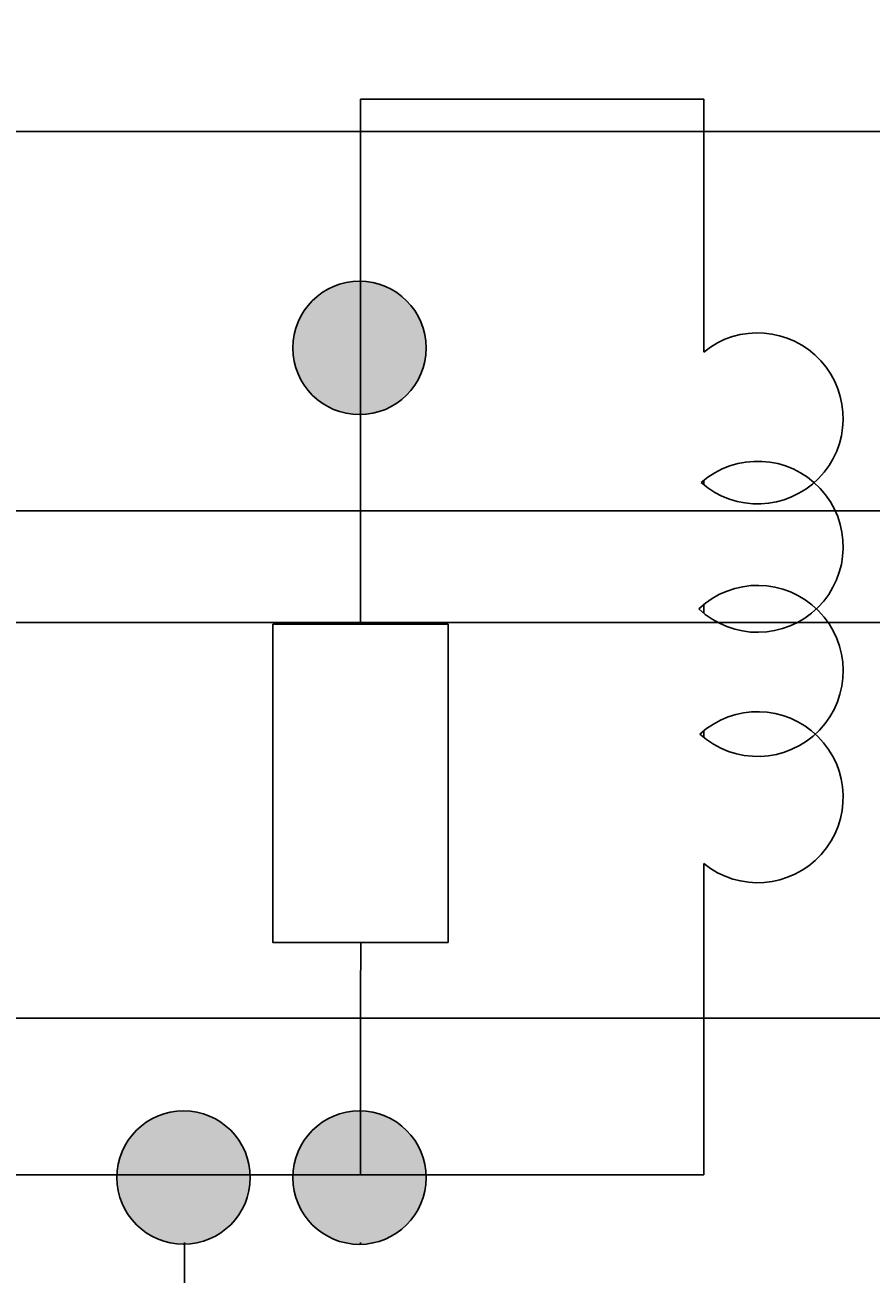
# Model space of a CAD drawing. Units: inches. Extents: x 35362 to 73946, y 43607 to 67532.
# Tile 134 of 134: x 69338 to 71350, y 58575 to 61547. Entities that reach past the tile are written whole.
import ezdxf

# ---------------------------------------------------------------- set-up
doc = ezdxf.new("R2010")
doc.units = ezdxf.units.IN
doc.header["$MEASUREMENT"] = 0
for name, color, linetype, lineweight in [('A-ANNO-DIMS', 2, 'Continuous', 18), ('E-SYMB', 1, 'Continuous', 25), ('E-SYMB-PATT', 1, 'Continuous', 13), ('E-WIRE', 3, 'Continuous', 25)]:
    doc.layers.add(name, color=color, linetype=linetype, lineweight=lineweight)
doc.styles.get("Standard").update_dxf_attribs({"font": 'arial.ttf'})
doc.dimstyles.get("Standard").update_dxf_attribs({"dimtxt": 0.18, "dimasz": 0.18, "dimexe": 0.18, "dimexo": 0.0625, "dimgap": 0.09, "dimtad": 0, "dimtih": 1, "dimtoh": 1, "dimdec": 4, "dimzin": 0, "dimdsep": 46, "dimtxsty": 'Standard', "dimcen": 0.09, "dimadec": 0, "dimazin": 0, "dimtfac": 1, "dimtdec": 4, "dimtofl": 0, "dimtmove": 0, "dimatfit": 3, "dimfxl": 1, "dimtolj": 1, "dimtzin": 0, "dimarcsym": 0})

# ---------------------------------------------------------------- blocks, each defined once
blk = doc.blocks.new('*D8')
at = {"layer": 'A-ANNO-DIMS', "color": 0, "lineweight": -2, "transparency": 16777216}
for p, q in [((66271.28651900003, 65771.51172800003), (73945.82566600003, 65771.51172800003)), ((73945.64566600005, 65771.33172800003), (73945.64566600005, 59737.03093663782)), ((73945.64566600005, 53702.36633900002), (73945.64566600005, 59736.66713036224)), ((72185.70816600003, 53702.18633900003), (73945.82566600003, 53702.18633900003))]:
    blk.add_line(p, q, dxfattribs=at)
at = {"layer": 'A-ANNO-DIMS', "color": 0, "transparency": 16777216}
for points in [[(73945.61566600006, 65771.33172800003), (73945.67566600005, 65771.33172800003), (73945.64566600005, 65771.51172800003)], [(73945.61566600006, 53702.36633900002), (73945.67566600005, 53702.36633900002), (73945.64566600005, 53702.18633900003)]]:
    blk.add_solid(points, dxfattribs=at)
at = {"layer": 'Defpoints', "color": 0, "transparency": 16777216}
for p in [(66271.22401900003, 65771.51172800003), (73945.64566600005, 65771.51172800003), (72185.64566600003, 53702.18633900003)]:
    blk.add_point(p, dxfattribs=at)
at = {"layer": 'A-ANNO-DIMS', "color": 0, "transparency": 16777216, "insert": (73945.64566600005, 59736.84903349999), "char_height": 0.18, "attachment_point": 5}
blk.add_mtext('\\A1;12069', dxfattribs=at)
blk = doc.blocks.new('*D10')
at = {"layer": 'A-ANNO-DIMS', "color": 0, "lineweight": -2, "transparency": 16777216}
for p, q in [((61240.96983600002, 59185.14395700003), (73945.82566600003, 59185.14395700003)), ((73945.64566600005, 59184.96395700003), (73945.64566600005, 56268.51827402935)), ((73945.64566600005, 53351.70866200003), (73945.64566600005, 56268.1543449707)), ((61240.96983600002, 53351.52866200003), (73945.82566600003, 53351.52866200003))]:
    blk.add_line(p, q, dxfattribs=at)
at = {"layer": 'A-ANNO-DIMS', "color": 0, "transparency": 16777216}
for points in [[(73945.61566600006, 59184.96395700003), (73945.67566600005, 59184.96395700003), (73945.64566600005, 59185.14395700003)], [(73945.61566600006, 53351.70866200003), (73945.67566600005, 53351.70866200003), (73945.64566600005, 53351.52866200003)]]:
    blk.add_solid(points, dxfattribs=at)
at = {"layer": 'Defpoints', "color": 0, "transparency": 16777216}
for p in [(61240.90733600002, 59185.14395700003), (61240.90733600002, 53351.52866200003), (73945.64566600005, 53351.52866200003)]:
    blk.add_point(p, dxfattribs=at)
at = {"layer": 'A-ANNO-DIMS', "color": 0, "transparency": 16777216, "insert": (73945.64566600005, 56268.33630949999), "char_height": 0.18, "attachment_point": 5}
blk.add_mtext('\\A1;5834', dxfattribs=at)
blk = doc.blocks.new('*D66')
at = {"layer": 'A-ANNO-DIMS', "color": 0, "lineweight": -2, "transparency": 16777216}
for p, q in [((67326.70224100004, 64127.44160800003), (73945.82566600003, 64127.44160800003)), ((73945.64566600005, 64127.26160800003), (73945.64566600005, 62710.54579452936)), ((73945.64566600005, 61293.46605200003), (73945.64566600005, 62710.1818654707)), ((67326.70224100004, 61293.28605200003), (73945.82566600003, 61293.28605200003))]:
    blk.add_line(p, q, dxfattribs=at)
at = {"layer": 'A-ANNO-DIMS', "color": 0, "transparency": 16777216}
for points in [[(73945.61566600006, 64127.26160800003), (73945.67566600005, 64127.26160800003), (73945.64566600005, 64127.44160800003)], [(73945.61566600006, 61293.46605200003), (73945.67566600005, 61293.46605200003), (73945.64566600005, 61293.28605200003)]]:
    blk.add_solid(points, dxfattribs=at)
at = {"layer": 'Defpoints', "color": 0, "transparency": 16777216}
for p in [(67326.63974100004, 64127.44160800003), (73945.64566600005, 64127.44160800003), (67326.63974100004, 61293.28605200003)]:
    blk.add_point(p, dxfattribs=at)
at = {"layer": 'A-ANNO-DIMS', "color": 0, "transparency": 16777216, "insert": (73945.64566600005, 62710.36383), "char_height": 0.18, "attachment_point": 5}
blk.add_mtext('\\A1;2834.2', dxfattribs=at)
blk = doc.blocks.new('*D69')
at = {"layer": 'A-ANNO-DIMS', "color": 0, "lineweight": -2, "transparency": 16777216}
for p, q in [((68320.870762, 60122.408832), (68320.870762, 67531.691728)), ((68321.050762, 67531.51172799998), (69913.30289879469, 67531.51172799998)), ((71506.482539, 67531.51172799998), (69914.23040220531, 67531.51172799998)), ((71506.662539, 59451.647447), (71506.662539, 67531.691728))]:
    blk.add_line(p, q, dxfattribs=at)
at = {"layer": 'A-ANNO-DIMS', "color": 0, "transparency": 16777216}
for points in [[(68321.050762, 67531.541728), (68321.050762, 67531.481728), (68320.870762, 67531.51172799998)], [(71506.482539, 67531.541728), (71506.482539, 67531.481728), (71506.662539, 67531.51172799998)]]:
    blk.add_solid(points, dxfattribs=at)
at = {"layer": 'Defpoints', "color": 0, "transparency": 16777216}
for p in [(71506.662539, 67531.51172799998), (68320.870762, 60122.346332), (71506.662539, 59451.584947)]:
    blk.add_point(p, dxfattribs=at)
at = {"layer": 'A-ANNO-DIMS', "color": 0, "transparency": 16777216, "insert": (69913.76665050001, 67531.51172799998), "char_height": 0.18, "attachment_point": 5}
blk.add_mtext('\\A1;3185.8', dxfattribs=at)
blk = doc.blocks.new('*D70')
at = {"layer": 'A-ANNO-DIMS', "color": 0, "lineweight": -2, "transparency": 16777216}
for p, q in [((60785.27513900002, 64923.75242000003), (73945.82566600003, 64923.75242000003)), ((73945.64566600005, 64923.57242000003), (73945.64566600005, 62054.63015302935)), ((73945.64566600005, 59185.32395700003), (73945.64566600005, 62054.26622397069)), ((61240.96983600002, 59185.14395700003), (73945.82566600003, 59185.14395700003))]:
    blk.add_line(p, q, dxfattribs=at)
at = {"layer": 'A-ANNO-DIMS', "color": 0, "transparency": 16777216}
for points in [[(73945.61566600006, 64923.57242000003), (73945.67566600005, 64923.57242000003), (73945.64566600005, 64923.75242000003)], [(73945.61566600006, 59185.32395700003), (73945.67566600005, 59185.32395700003), (73945.64566600005, 59185.14395700003)]]:
    blk.add_solid(points, dxfattribs=at)
at = {"layer": 'Defpoints', "color": 0, "transparency": 16777216}
for p in [(60785.21263900002, 64923.75242000003), (73945.64566600005, 64923.75242000003), (61240.90733600002, 59185.14395700003)]:
    blk.add_point(p, dxfattribs=at)
at = {"layer": 'A-ANNO-DIMS', "color": 0, "transparency": 16777216, "insert": (73945.64566600005, 62054.44818849999), "char_height": 0.18, "attachment_point": 5}
blk.add_mtext('\\A1;5738.6', dxfattribs=at)
blk = doc.blocks.new('*D71')
at = {"layer": 'A-ANNO-DIMS', "color": 0, "lineweight": -2, "transparency": 16777216}
for p, q in [((63159.24181700003, 64828.55626700002), (73945.82566600003, 64828.55626700002)), ((73945.64566600005, 64828.37626700002), (73945.64566600005, 62007.03207652936)), ((73945.64566600005, 59185.32395700003), (73945.64566600005, 62006.6681474707)), ((61240.96983600002, 59185.14395700003), (73945.82566600003, 59185.14395700003))]:
    blk.add_line(p, q, dxfattribs=at)
at = {"layer": 'A-ANNO-DIMS', "color": 0, "transparency": 16777216}
for points in [[(73945.61566600006, 64828.37626700002), (73945.67566600005, 64828.37626700002), (73945.64566600005, 64828.55626700002)], [(73945.61566600006, 59185.32395700003), (73945.67566600005, 59185.32395700003), (73945.64566600005, 59185.14395700003)]]:
    blk.add_solid(points, dxfattribs=at)
at = {"layer": 'Defpoints', "color": 0, "transparency": 16777216}
for p in [(63159.17931700003, 64828.55626700002), (73945.64566600005, 64828.55626700002), (61240.90733600002, 59185.14395700003)]:
    blk.add_point(p, dxfattribs=at)
at = {"layer": 'A-ANNO-DIMS', "color": 0, "transparency": 16777216, "insert": (73945.64566600005, 62006.85011199999), "char_height": 0.18, "attachment_point": 5}
blk.add_mtext('\\A1;5643.4', dxfattribs=at)
blk = doc.blocks.new('*D113')
at = {"layer": 'A-ANNO-DIMS', "color": 0, "lineweight": -2, "transparency": 16777216}
for p, q in [((53526.13474100003, 60391.71935800003), (73945.82566600003, 60391.71935800003)), ((73945.64566600005, 60391.53935800003), (73945.64566600005, 60259.19182863781)), ((73945.64566600005, 60126.48049300003), (73945.64566600005, 60258.82802236224)), ((53705.42262200003, 60126.30049300003), (73945.82566600003, 60126.30049300003))]:
    blk.add_line(p, q, dxfattribs=at)
at = {"layer": 'A-ANNO-DIMS', "color": 0, "transparency": 16777216}
for points in [[(73945.61566600006, 60391.53935800003), (73945.67566600005, 60391.53935800003), (73945.64566600005, 60391.71935800003)], [(73945.61566600006, 60126.48049300003), (73945.67566600005, 60126.48049300003), (73945.64566600005, 60126.30049300003)]]:
    blk.add_solid(points, dxfattribs=at)
at = {"layer": 'Defpoints', "color": 0, "transparency": 16777216}
for p in [(53526.07224100003, 60391.71935800003), (73945.64566600005, 60391.71935800003), (53705.36012200003, 60126.30049300003)]:
    blk.add_point(p, dxfattribs=at)
at = {"layer": 'A-ANNO-DIMS', "color": 0, "transparency": 16777216, "insert": (73945.64566600005, 60259.00992549999), "char_height": 0.18, "attachment_point": 5}
blk.add_mtext('\\A1;265.4', dxfattribs=at)

msp = doc.modelspace()

# ---------------------------------------------------------------- hatches: boundary and pattern name
at = {"layer": 'E-SYMB-PATT'}
h = msp.add_hatch(color=256, dxfattribs=at)
h.dxf.hatch_style = 1
h.paths.add_polyline_path([(70135.80528894292, 60937.4800173882, 0.4183931940818975), (69974.93949760578, 60778.89023200967, 0.4183931940818975), (70135.80528894292, 60620.30044663113)])
h.paths.add_polyline_path([(70135.80528894292, 60937.4800173882), (70135.80528894292, 60620.30044663113, 0.4100462469397049), (70292.15127038094, 60778.89023200967, 0.4100462469397049)])
h = msp.add_hatch(color=256, dxfattribs=at)
h.dxf.hatch_style = 1
h.paths.add_polyline_path([(69717.45127656072, 58965.3185751958, 0.4183931940818975), (69556.58548522356, 58806.72878981727, 0.4183931940818975), (69717.45127656072, 58648.13900443873)])
h.paths.add_polyline_path([(69717.45127656072, 58965.3185751958), (69717.45127656072, 58648.13900443873, 0.4100462469397049), (69873.79725799873, 58806.72878981727, 0.4100462469397049)])
h = msp.add_hatch(color=256, dxfattribs=at)
h.dxf.hatch_style = 1
h.paths.add_polyline_path([(70135.80528894292, 58965.03303138048, 0.4183931940818975), (69974.93949760577, 58806.44324600194, 0.4183931940818975), (70135.80528894292, 58647.8534606234)])
h.paths.add_polyline_path([(70135.80528894292, 58965.03303138048), (70135.80528894292, 58647.8534606234, 0.4100462469397049), (70292.15127038091, 58806.44324600194, 0.4100462469397049)])

# ---------------------------------------------------------------- linework, layer by layer
at = {"layer": 'E-SYMB'}
for p, q in [((70951.91702453484, 60769.1106295505), (70951.91702453484, 61035.31232071571)), ((70131.22999091068, 60937.47921697288), (70131.22999091068, 60936.79299371184)), ((70135.80528894292, 60624.77159211603), (70135.80528894292, 60620.30044663113)), ((70135.80528894292, 60538.65863418842), (70135.80528894292, 60122.34633153839)), ((70951.91702453484, 60463.84216359539), (70951.91702453484, 60453.6665256447)), ((70951.91702453484, 60168.74933559101), (70951.91702453484, 60148.39805968959)), ((70951.91702453484, 59868.56864057082), (70951.91702453484, 59853.30523168521)), ((70951.91702453484, 59553.124536665), (70951.91702453484, 59355.50749272094)), ((70135.80528894292, 59232.80970853629), (70136.39879188087, 59365.72803786365)), ((70951.91702453484, 59355.50749272094), (70951.91702453484, 59232.80970853629)), ((69712.87597852846, 58965.31777478048), (69712.87597852846, 58964.63155151943)), ((70131.22999091067, 58965.03223096516), (70131.22999091067, 58964.34600770412)), ((69717.45127656072, 58652.61014992363), (69717.45127656072, 58648.13900443873)), ((70135.80528894292, 58652.32460610831), (70135.80528894292, 58647.8534606234))]:
    msp.add_line(p, q, dxfattribs=at)
msp.add_lwpolyline([(69927.32366271509, 60122.34633153839), (70344.25478159498, 60122.34633153839), (70344.25478159498, 59365.72803786365), (69927.32366271509, 59365.72803786365)], close=True, dxfattribs=at)
for centre in [(70133.54538399336, 60778.89023200967), (69715.19137161114, 58806.72878981727), (70133.54538399335, 58806.44324600194)]:
    msp.add_circle(centre, 158.6058863875805, dxfattribs=at)
for centre, start, end in [((71080.24668337766, 60611.3885775976), 228.6473573753378, 129.133331426897), ((71080.24668337766, 60306.12011164249), 226.5217351845933, 131.3526426246621), ((71080.24668337766, 60011.02728363811), 227.5737684206446, 133.4782648154067), ((71080.24668337766, 59710.84658861791), 230.866668573103, 132.4262315793553)]:
    msp.add_arc(centre, 203.3340773479672, start, end, dxfattribs=at)
at = {"layer": 'E-WIRE'}
for p, q in [((70135.80528894292, 60955.44019388535), (70135.80528894292, 61370.18605940839)), ((70135.80528894292, 61370.18605940839), (70951.91702453484, 61370.18605940839)), ((70951.91702453484, 61370.18605940839), (70951.91702453484, 61035.31232071571)), ((70135.80528894292, 60538.65863418842), (70135.80528894292, 60955.44019388535)), ((70135.80528894292, 59232.80970853629), (70135.80528894292, 58812.79476317562)), ((70951.91702453484, 58812.79476317562), (70951.91702453484, 59232.80970853629)), ((70135.80528894292, 58812.79476317562), (68677.76702326702, 58813.78993424351)), ((70135.80528894292, 58812.79476317562), (70951.91702453484, 58812.79476317562)), ((69717.45127656072, 58414.54422497431), (69717.45127656072, 58648.13900443873))]:
    msp.add_line(p, q, dxfattribs=at)

# ---------------------------------------------------------------- dimensions: what is measured, and where the dimension line sits
at = {"layer": 'A-ANNO-DIMS'}
dim = msp.add_linear_dim(base=(71506.662539, 67531.51172799998), p1=(68320.870762, 60122.346332), p2=(71506.662539, 59451.584947), dimstyle='Standard', override={"dimdec": 1, "dimlfac": 1, "dimrnd": 0, "dimzin": 0, "dimdsep": 46, "dimlunit": 2}, dxfattribs=at)
dim.commit()
dim.dimension.update_dxf_attribs({"geometry": '*D69', "text_midpoint": (69913.76665050001, 67531.51172799998)})
for base, p1, p2, override, picture, middle in [((73945.64566600005, 65771.51172800003), (72185.645666, 53702.186339), (66271.224019, 65771.51172799998), {"dimdec": 0, "dimlfac": 1, "dimrnd": 0, "dimzin": 0, "dimdsep": 46, "dimlunit": 2}, '*D8', (73945.64566600005, 59736.84903349999)), ((73945.64566600005, 64923.75242000003), (61240.907336, 59185.14395699999), (60785.21263899999, 64923.75241999999), {"dimdec": 1, "dimlfac": 1, "dimrnd": 0, "dimzin": 0, "dimdsep": 46, "dimlunit": 2}, '*D70', (73945.64566600005, 62054.44818849999)), ((73945.64566600005, 64828.55626700002), (61240.907336, 59185.14395699999), (63159.179317, 64828.556267), {"dimdec": 1, "dimlfac": 1, "dimrnd": 0, "dimzin": 0, "dimdsep": 46, "dimlunit": 2}, '*D71', (73945.64566600005, 62006.85011199999)), ((73945.64566600005, 64127.44160800003), (67326.639741, 61293.286052), (67326.639741, 64127.44160799999), {"dimdec": 1, "dimlfac": 1, "dimrnd": 0, "dimzin": 0, "dimdsep": 46, "dimlunit": 2}, '*D66', (73945.64566600005, 62710.36383)), ((73945.64566600005, 60391.71935800003), (53705.36012199999, 60126.300493), (53526.072241, 60391.719358), {"dimdec": 1, "dimlfac": 1, "dimrnd": 0, "dimzin": 0, "dimdsep": 46, "dimlunit": 2}, '*D113', (73945.64566600005, 60259.00992549999)), ((73945.64566600005, 53351.52866200003), (61240.907336, 59185.14395699999), (61240.907336, 53351.52866199999), {"dimdec": 0, "dimlfac": 1, "dimrnd": 0, "dimzin": 0, "dimdsep": 46, "dimlunit": 2}, '*D10', (73945.64566600005, 56268.33630949999))]:
    dim = msp.add_linear_dim(base=base, p1=p1, p2=p2, angle=90, dimstyle='Standard', override=override, dxfattribs=at)
    dim.commit()
    dim.dimension.update_dxf_attribs({"geometry": picture, "text_midpoint": middle})

doc.saveas('drawing.dxf')
